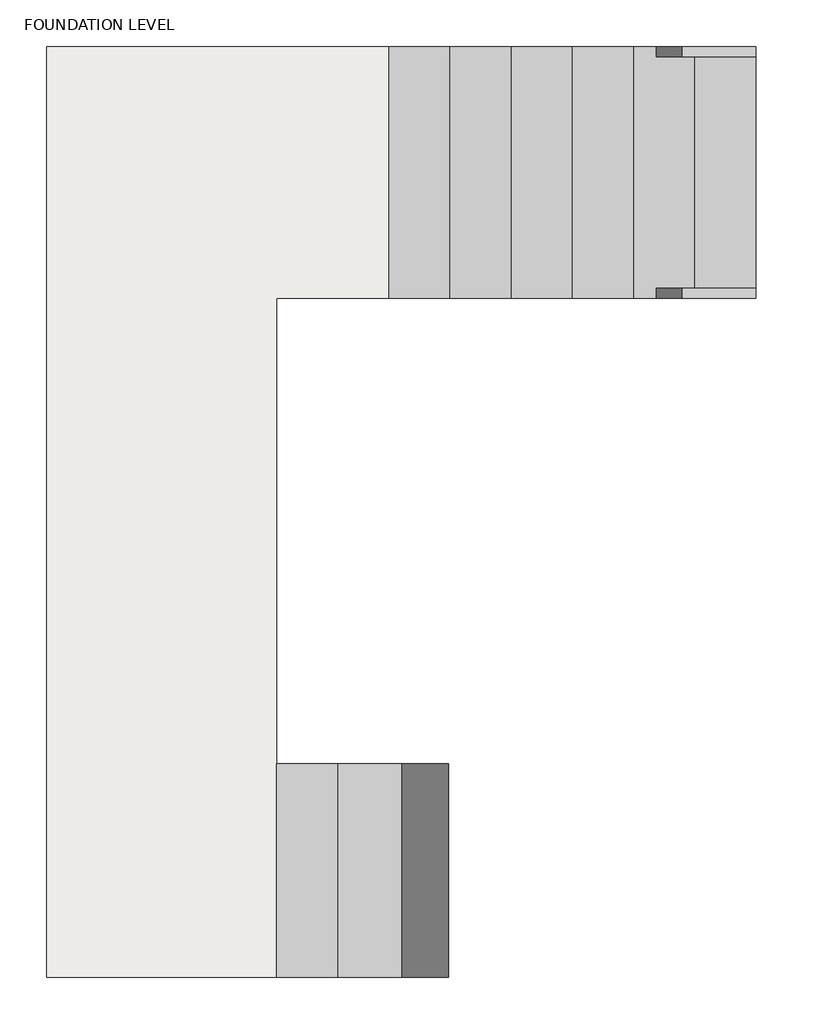
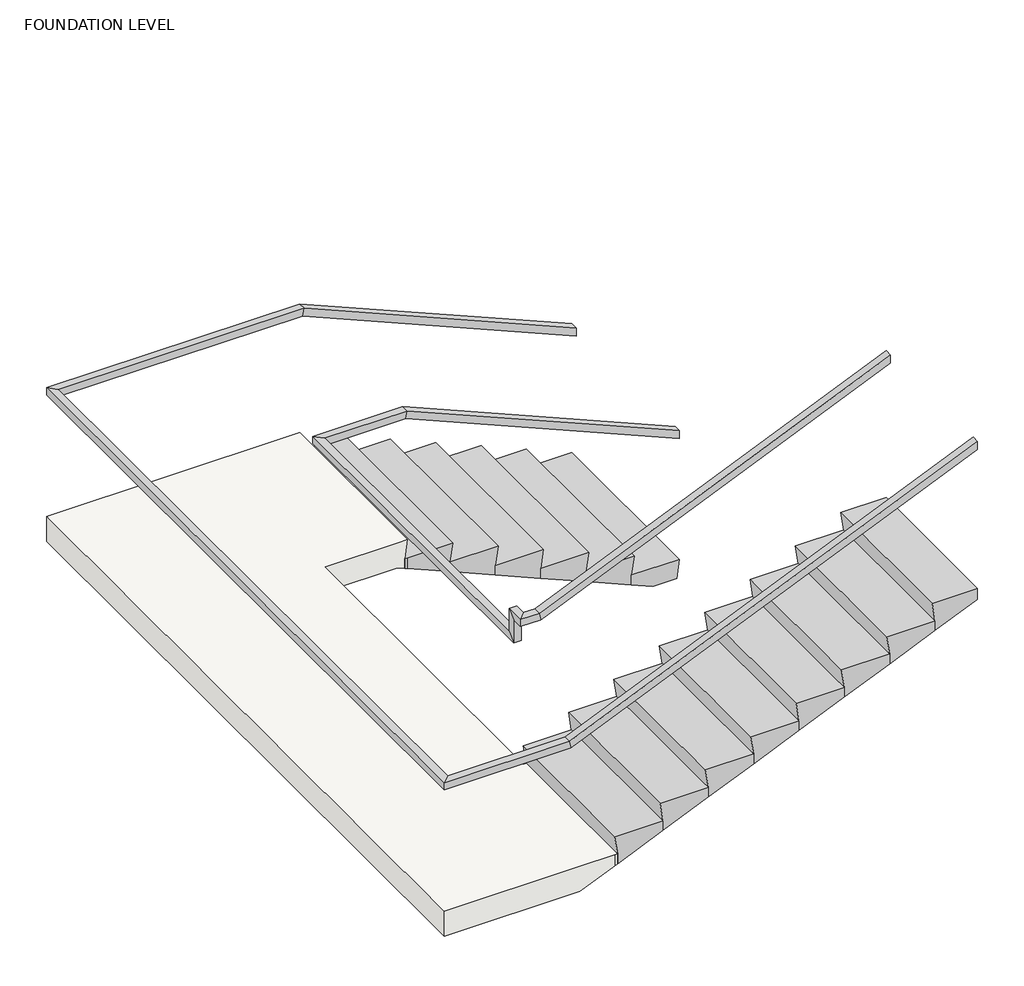
# One storey: 2 railings, 2 stair flights, 1 slab.
"""IFC4 building model written with IfcOpenShell, lengths in millimetres."""

from ifc_helpers import new_model, si_unit, origin, place, context, project, spatial, faceted_brep, element, save

model = new_model("IFC4")

# Units and contexts
model_context = context("Model", 3, world=origin())
ifc_project = project(units=[si_unit("LENGTHUNIT", "METRE", prefix="MILLI")], contexts=[model_context])

# Site, building, storey
site = spatial("IfcSite", under=ifc_project)
building = spatial("IfcBuilding", under=site)
storey = spatial("IfcBuildingStorey", under=building, Name="FOUNDATION LEVEL", Elevation=-3487.2011518)

# Railings
placement = place(None, origin())
element("IfcRailing", 1, ObjectType="Handrail", at=placement, inside=storey, context=model_context, shape_type="Brep", body=[
    faceted_brep([(6487.8258195, 16426.305974, -2442.6261518), (6487.8258195, 16426.305974, -2497.8651705), (6487.8258195, 16477.105974, -2497.8651705), (6487.8258195, 16477.105974, -2442.6261518), (4659.0258195, 16426.305974, -1661.5761518), (4648.6320197, 16426.305974, -1712.3761518), (4648.6320197, 16477.105974, -1712.3761518), (4659.0258195, 16477.105974, -1661.5761518), (3008.0258195, 16426.305974, -1661.5761518), (3008.0258195, 16426.305974, -1712.3761518), (2957.2258195, 16477.105974, -1712.3761518), (2957.2258195, 16477.105974, -1661.5761518), (3008.0258195, 11896.1816424, -1661.5761518), (3008.0258195, 11896.1816424, -1712.3761518), (2957.2258195, 11845.3816424, -1712.3761518), (2957.2258195, 11845.3816424, -1661.5761518), (3797.8923097, 11896.1816424, -1661.5761518), (3808.2861096, 11896.1816424, -1712.3761518), (3808.2861096, 11845.3816424, -1712.3761518), (3797.8923097, 11845.3816424, -1661.5761518), (6541.0923097, 11896.1816424, -490.0011518), (6541.0923097, 11845.3816424, -490.0011518), (6541.0923097, 11845.3816424, -545.2401705), (6541.0923097, 11896.1816424, -545.2401705)], [[[0, 1, 2, 3]], [[1, 0, 4, 5]], [[2, 1, 5, 6]], [[3, 2, 6, 7]], [[0, 3, 7, 4]], [[5, 4, 8, 9]], [[6, 5, 9, 10]], [[7, 6, 10, 11]], [[4, 7, 11, 8]], [[9, 8, 12, 13]], [[10, 9, 13, 14]], [[11, 10, 14, 15]], [[8, 11, 15, 12]], [[13, 12, 16, 17]], [[14, 13, 17, 18]], [[15, 14, 18, 19]], [[12, 15, 19, 16]], [[20, 21, 22, 23]], [[17, 16, 20, 23]], [[18, 17, 23, 22]], [[19, 18, 22, 21]], [[16, 19, 21, 20]]]),
])
element("IfcRailing", 2, ObjectType="Handrail", at=placement, inside=storey, context=model_context, shape_type="Brep", body=[
    faceted_brep([(6487.8258195, 15223.6852874, -2442.6261518), (6487.8258195, 15223.6852874, -2497.8651705), (6487.8258195, 15274.4852874, -2497.8651705), (6487.8258195, 15274.4852874, -2442.6261518), (4659.0258195, 15223.6852874, -1661.5761518), (4648.6320197, 15223.6852874, -1712.3761518), (4648.6320197, 15274.4852874, -1712.3761518), (4659.0258195, 15274.4852874, -1661.5761518), (4102.6923097, 15223.6852874, -1661.5761518), (4102.6923097, 15223.6852874, -1712.3761518), (4051.8923097, 15274.4852874, -1712.3761518), (4051.8923097, 15274.4852874, -1661.5761518), (4102.6923097, 12985.9409784, -1661.5761518), (4102.6923097, 12935.1409784, -1712.3761518), (4051.8923097, 12935.1409784, -1712.3761518), (4051.8923097, 12985.9409784, -1661.5761518), (4102.6923097, 12985.9409784, -1498.8574018), (4102.6923097, 12935.1409784, -1549.6574018), (4051.8923097, 12935.1409784, -1549.6574018), (4051.8923097, 12985.9409784, -1498.8574018), (4102.6923097, 12909.7409784, -1498.8574018), (4102.6923097, 12909.7409784, -1549.6574018), (4051.8923097, 12858.9409784, -1549.6574018), (4051.8923097, 12858.9409784, -1498.8574018), (4178.8923097, 12909.7409784, -1498.8574018), (4189.2861096, 12909.7409784, -1549.6574018), (4189.2861096, 12858.9409784, -1549.6574018), (4178.8923097, 12858.9409784, -1498.8574018), (6541.0923097, 12909.7409784, -490.0011518), (6541.0923097, 12858.9409784, -490.0011518), (6541.0923097, 12858.9409784, -545.2401705), (6541.0923097, 12909.7409784, -545.2401705)], [[[0, 1, 2, 3]], [[1, 0, 4, 5]], [[2, 1, 5, 6]], [[3, 2, 6, 7]], [[0, 3, 7, 4]], [[5, 4, 8, 9]], [[6, 5, 9, 10]], [[7, 6, 10, 11]], [[4, 7, 11, 8]], [[9, 8, 12, 13]], [[10, 9, 13, 14]], [[11, 10, 14, 15]], [[8, 11, 15, 12]], [[13, 12, 16, 17]], [[14, 13, 17, 18]], [[15, 14, 18, 19]], [[12, 15, 19, 16]], [[17, 16, 20, 21]], [[18, 17, 21, 22]], [[19, 18, 22, 23]], [[16, 19, 23, 20]], [[21, 20, 24, 25]], [[22, 21, 25, 26]], [[23, 22, 26, 27]], [[20, 23, 27, 24]], [[28, 29, 30, 31]], [[25, 24, 28, 31]], [[26, 25, 31, 30]], [[27, 26, 30, 29]], [[24, 27, 29, 28]]]),
])

# Slab
element("IfcSlab", 3, ObjectType="7\" Thickness", at=placement, inside=storey, context=model_context, shape_type="Brep", body=[
    faceted_brep([(4659.0258195, 16477.105974, -2575.9761518), (4659.0258195, 15223.6852874, -2575.9761518), (4639.9758195, 15223.6852874, -2706.1511518), (4639.9758195, 16477.105974, -2706.1511518), (2957.2258195, 16477.105974, -2575.9761518), (2957.2258195, 11845.3816424, -2575.9761518), (3867.1052912, 11845.3816424, -2575.9761518), (4102.6923097, 11845.3816424, -2575.9761518), (4121.7423097, 11845.3816424, -2575.9761518), (4121.7423097, 12909.7409784, -2575.9761518), (4102.6923097, 12909.7409784, -2575.9761518), (4102.6923097, 15223.6852874, -2575.9761518), (4589.812838, 15223.6852874, -2575.9761518), (4589.812838, 16477.105974, -2575.9761518), (4639.9758195, 15223.6852874, -2775.1999252), (4639.9758195, 16477.105974, -2775.1999252), (4589.812838, 16477.105974, -2753.7761518), (2957.2258195, 16477.105974, -2753.7761518), (2957.2258195, 11845.3816424, -2753.7761518), (3867.1052912, 11845.3816424, -2753.7761518), (4102.6923097, 11845.3816424, -2653.1608627), (4121.7423097, 11845.3816424, -2645.0249252), (4121.7423097, 12909.7409784, -2645.0249252), (4102.6923097, 12909.7409784, -2653.1608627), (4102.6923097, 12909.7409784, -2753.7761518), (4102.6923097, 15223.6852874, -2753.7761518), (4589.812838, 15223.6852874, -2753.7761518), (3867.1052912, 12909.7409784, -2753.7761518)], [[[0, 1, 2, 3]], [[4, 5, 6, 7, 8, 9, 10, 11, 12, 1, 0, 13]], [[3, 2, 14, 15]], [[0, 3, 15, 16, 17, 4, 13]], [[5, 4, 17, 18]], [[5, 18, 19, 20, 7, 6]], [[8, 7, 20, 21]], [[9, 8, 21, 22]], [[10, 9, 22, 23]], [[11, 10, 23, 24, 25]], [[2, 1, 12, 11, 25, 26, 14]], [[24, 27, 19, 18, 17, 16, 26, 25]], [[27, 24, 23]], [[26, 16, 15, 14]], [[19, 27, 23, 22, 21, 20]]]),
])

# Stair flights
element("IfcStairFlight", 4, ObjectType="3/4\" Nosing", at=placement, inside=storey, context=model_context, shape_type="Brep", body=[
    faceted_brep([(6487.8258195, 16477.105974, -3357.0261518), (6487.8258195, 15223.6852874, -3357.0261518), (6468.7758195, 15223.6852874, -3487.2011518), (6468.7758195, 16477.105974, -3487.2011518), (6163.9758195, 16477.105974, -3357.0261518), (6163.9758195, 15223.6852874, -3357.0261518), (6163.9758195, 15223.6852874, -3426.0749252), (6307.1006429, 15223.6852874, -3487.2011518), (6307.1006429, 16477.105974, -3487.2011518), (6163.9758195, 16477.105974, -3426.0749252), (6183.0258195, 15223.6852874, -3226.8511518), (6183.0258195, 16477.105974, -3226.8511518), (5859.1758195, 16477.105974, -3226.8511518), (5859.1758195, 15223.6852874, -3226.8511518), (5859.1758195, 15223.6852874, -3295.8999252), (5859.1758195, 16477.105974, -3295.8999252), (5878.2258195, 15223.6852874, -3096.6761518), (5878.2258195, 16477.105974, -3096.6761518), (5554.3758195, 16477.105974, -3096.6761518), (5554.3758195, 15223.6852874, -3096.6761518), (5554.3758195, 15223.6852874, -3165.7249252), (5554.3758195, 16477.105974, -3165.7249252), (5573.4258195, 15223.6852874, -2966.5011518), (5573.4258195, 16477.105974, -2966.5011518), (5249.5758195, 16477.105974, -2966.5011518), (5249.5758195, 15223.6852874, -2966.5011518), (5249.5758195, 15223.6852874, -3035.5499252), (5249.5758195, 16477.105974, -3035.5499252), (5268.6258195, 15223.6852874, -2836.3261518), (5268.6258195, 16477.105974, -2836.3261518), (4944.7758195, 16477.105974, -2836.3261518), (4944.7758195, 15223.6852874, -2836.3261518), (4944.7758195, 15223.6852874, -2905.3749252), (4944.7758195, 16477.105974, -2905.3749252), (4639.9758195, 15223.6852874, -2706.1511518), (4659.0258195, 15223.6852874, -2706.1511518), (4963.8258195, 15223.6852874, -2706.1511518), (4963.8258195, 16477.105974, -2706.1511518), (4659.0258195, 16477.105974, -2706.1511518), (4639.9758195, 16477.105974, -2706.1511518), (4639.9758195, 15223.6852874, -2775.1999252), (4659.0258195, 15223.6852874, -2783.3358627), (4659.0258195, 16477.105974, -2783.3358627), (4639.9758195, 16477.105974, -2775.1999252)], [[[0, 1, 2, 3]], [[1, 0, 4, 5]], [[1, 5, 6, 7, 2]], [[4, 0, 3, 8, 9]], [[10, 11, 12, 13]], [[10, 13, 14, 6, 5]], [[12, 11, 4, 9, 15]], [[5, 4, 11, 10]], [[16, 17, 18, 19]], [[16, 19, 20, 14, 13]], [[18, 17, 12, 15, 21]], [[13, 12, 17, 16]], [[22, 23, 24, 25]], [[22, 25, 26, 20, 19]], [[24, 23, 18, 21, 27]], [[19, 18, 23, 22]], [[28, 29, 30, 31]], [[28, 31, 32, 26, 25]], [[30, 29, 24, 27, 33]], [[25, 24, 29, 28]], [[34, 35, 36, 37, 38, 39]], [[35, 34, 40, 41]], [[38, 37, 30, 33, 42]], [[34, 39, 43, 40]], [[31, 30, 37, 36]], [[3, 2, 7, 8]], [[8, 7, 6, 14, 20, 26, 32, 41, 40, 43, 42, 33, 27, 21, 15, 9]], [[36, 35, 41, 32, 31]], [[39, 38, 42, 43]]]),
])
element("IfcStairFlight", 5, ObjectType="3/4\" Nosing", at=placement, inside=storey, context=model_context, shape_type="Brep", body=[
    faceted_brep([(4102.6923097, 11845.3816424, -2445.8011518), (4102.6923097, 12909.7409784, -2445.8011518), (4121.7423097, 12909.7409784, -2575.9761518), (4121.7423097, 11845.3816424, -2575.9761518), (4426.5423097, 11845.3816424, -2445.8011518), (4426.5423097, 12909.7409784, -2445.8011518), (4426.5423097, 12909.7409784, -2514.8499252), (4121.7423097, 12909.7409784, -2645.0249252), (4121.7423097, 11845.3816424, -2645.0249252), (4426.5423097, 11845.3816424, -2514.8499252), (4407.4923097, 12909.7409784, -2315.6261518), (4407.4923097, 11845.3816424, -2315.6261518), (4731.3423097, 11845.3816424, -2315.6261518), (4731.3423097, 12909.7409784, -2315.6261518), (4731.3423097, 12909.7409784, -2384.6749252), (4731.3423097, 11845.3816424, -2384.6749252), (4712.2923097, 12909.7409784, -2185.4511518), (4712.2923097, 11845.3816424, -2185.4511518), (5036.1423097, 11845.3816424, -2185.4511518), (5036.1423097, 12909.7409784, -2185.4511518), (5036.1423097, 12909.7409784, -2254.4999252), (5036.1423097, 11845.3816424, -2254.4999252), (5017.0923097, 12909.7409784, -2055.2761518), (5017.0923097, 11845.3816424, -2055.2761518), (5340.9423097, 11845.3816424, -2055.2761518), (5340.9423097, 12909.7409784, -2055.2761518), (5340.9423097, 12909.7409784, -2124.3249252), (5340.9423097, 11845.3816424, -2124.3249252), (5321.8923097, 12909.7409784, -1925.1011518), (5321.8923097, 11845.3816424, -1925.1011518), (5645.7423097, 11845.3816424, -1925.1011518), (5645.7423097, 12909.7409784, -1925.1011518), (5645.7423097, 12909.7409784, -1994.1499252), (5645.7423097, 11845.3816424, -1994.1499252), (5626.6923097, 12909.7409784, -1794.9261518), (5626.6923097, 11845.3816424, -1794.9261518), (5950.5423097, 11845.3816424, -1794.9261518), (5950.5423097, 12909.7409784, -1794.9261518), (5950.5423097, 12909.7409784, -1863.9749252), (5950.5423097, 11845.3816424, -1863.9749252), (5931.4923097, 12909.7409784, -1664.7511518), (5931.4923097, 11845.3816424, -1664.7511518), (6255.3423097, 11845.3816424, -1664.7511518), (6255.3423097, 12909.7409784, -1664.7511518), (6255.3423097, 12909.7409784, -1733.7999252), (6255.3423097, 11845.3816424, -1733.7999252), (6236.2923097, 12909.7409784, -1534.5761518), (6236.2923097, 11845.3816424, -1534.5761518), (6541.0923097, 11845.3816424, -1534.5761518), (6541.0923097, 12909.7409784, -1534.5761518), (6541.0923097, 12909.7409784, -1611.7608627), (6541.0923097, 11845.3816424, -1611.7608627)], [[[0, 1, 2, 3]], [[1, 0, 4, 5]], [[1, 5, 6, 7, 2]], [[3, 2, 7, 8]], [[4, 0, 3, 8, 9]], [[10, 11, 12, 13]], [[10, 13, 14, 6, 5]], [[12, 11, 4, 9, 15]], [[11, 10, 5, 4]], [[16, 17, 18, 19]], [[16, 19, 20, 14, 13]], [[18, 17, 12, 15, 21]], [[17, 16, 13, 12]], [[22, 23, 24, 25]], [[22, 25, 26, 20, 19]], [[24, 23, 18, 21, 27]], [[23, 22, 19, 18]], [[28, 29, 30, 31]], [[28, 31, 32, 26, 25]], [[30, 29, 24, 27, 33]], [[29, 28, 25, 24]], [[34, 35, 36, 37]], [[34, 37, 38, 32, 31]], [[36, 35, 30, 33, 39]], [[35, 34, 31, 30]], [[40, 41, 42, 43]], [[40, 43, 44, 38, 37]], [[42, 41, 36, 39, 45]], [[41, 40, 37, 36]], [[46, 47, 48, 49]], [[46, 49, 50, 44, 43]], [[48, 47, 42, 45, 51]], [[49, 48, 51, 50]], [[47, 46, 43, 42]], [[7, 6, 14, 20, 26, 32, 38, 44, 50, 51, 45, 39, 33, 27, 21, 15, 9, 8]]]),
])

save(model, "model.ifc")

# Revit data of these elements
# Grids (mm)
#   "1": line (-25501.549, 19004.013) -> (-25501.549, -9342.431)
#   "2": line (-20777.149, 18911.845) -> (-20777.149, -9434.599)
#   "3": line (-16357.549, 19081.95) -> (-16357.549, -9264.494)
#   "4": line (-11785.549, 19205.664) -> (-11785.549, -9140.781)
#   "5": line (-7518.349, 19112.879) -> (-7518.349, -9233.565)
#   "6": line (-2946.349, 19128.343) -> (-2946.349, -9218.101)
#   "7": line (1625.651, 18927.309) -> (1625.651, -9419.135)
#   "8": line (6197.651, 19128.343) -> (6197.651, -9218.101)
#   "15": line (-27431.844, 16916.969) -> (8940.851, 16916.969)
#   "16": line (-27431.844, 11430.569) -> (8940.851, 11430.569)
#   "17": line (-27431.844, 7772.969) -> (8940.851, 7772.969)
#   "18": line (-27431.844, 2896.169) -> (8940.851, 2896.169)
#   "19": line (-27431.844, -761.431) -> (8940.851, -761.431)
#   "20": line (-27431.844, -6247.831) -> (8940.851, -6247.831)
# Type "Handrail"
#   Assembly Code = "C2010400"
#   built-in parameter 1008612 = 0.0416667 (stored number, unit not read)
#   built-in parameter 1008611 = 0.0416667 (stored number, unit not read)
#   built-in parameter 1008609 = 0.333333 (stored number, unit not read)
#   built-in parameter 1008604 = 0.166667 (stored number, unit not read)
#   built-in parameter 1008603 = 0.166667 (stored number, unit not read)
#   Railing Height = 3' - 0"
#   built-in parameter 1008630 = 2
#   built-in parameter 1008610 = 2
#   built-in parameter 1008618 = Baluster - Square : 3/4"
# Elements 1, 2 (IfcRailing, "Handrail")
#   Phase Created = New Construction
# Element 3 (IfcSlab, "7\" Thickness")
#   Phase Created = New Construction
#   Materials on its faces: "Concrete, Cast-in-Place gray"
# Elements 4, 5 (IfcStairFlight, "3/4\" Nosing")
#   Phase Created = New Construction
#   Materials on its faces: "Concrete, Cast-in-Place gray"
# Materials
#   "Concrete, Cast-in-Place gray": class "Concrete", colour RGB 192 192 192, transparency 0, Description = "Cast-in-place concrete", Cost = 0
